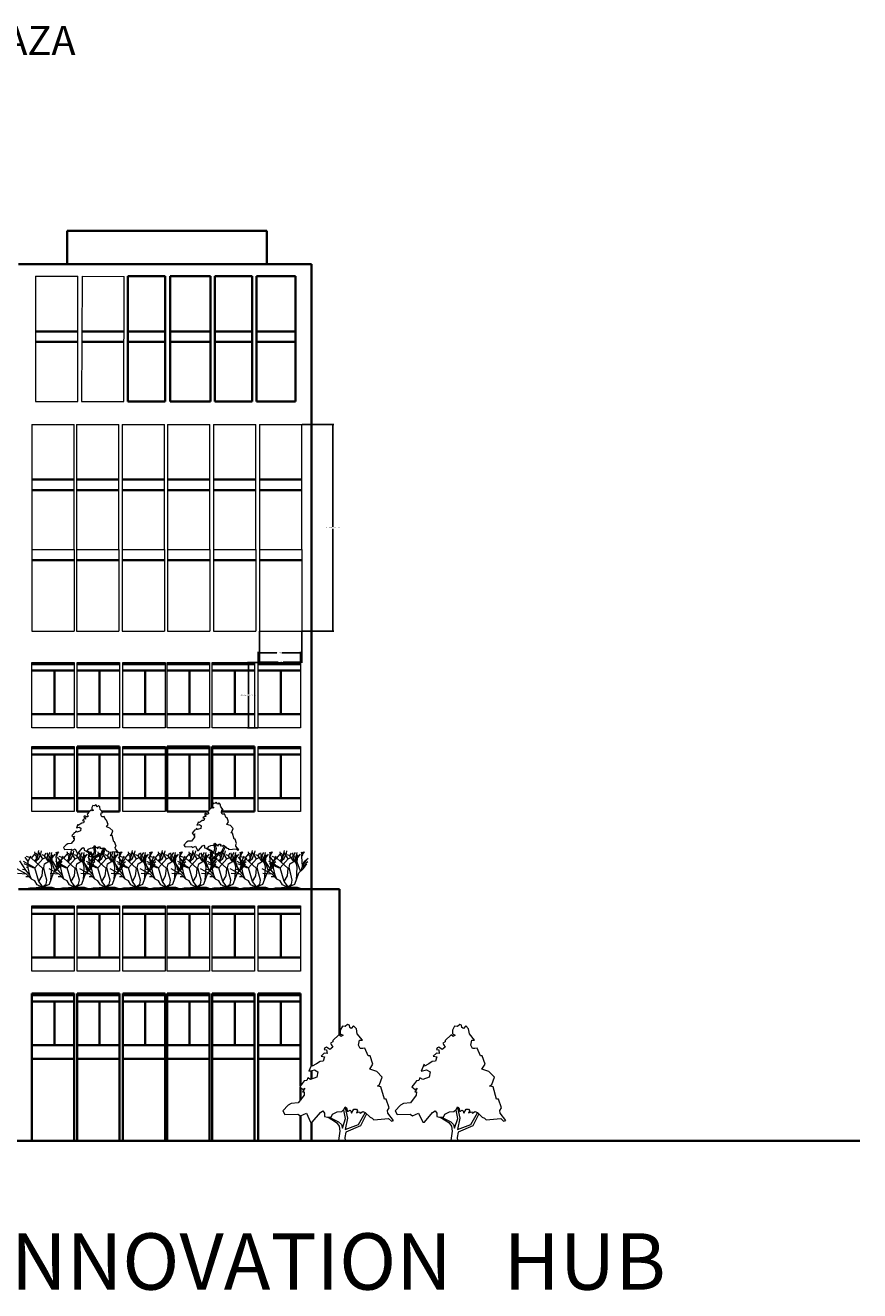
# Model space of a CAD drawing. Units: inches. Extents: x -362 to 223, y -437 to 70.
# Tile 5 of 5: x 67 to 223, y -166 to 70. Entities that reach past the tile are written whole.
import ezdxf

# ---------------------------------------------------------------- set-up
doc = ezdxf.new("R2010")
doc.units = ezdxf.units.IN
doc.header["$MEASUREMENT"] = 0
for name, color, linetype, lineweight in [('A-ANNO-DIMS', 2, 'Continuous', 18), ('A-ANNO-TEXT', 7, 'Continuous', 25), ('A-ELEV', 7, 'Continuous', 35), ('A-GLAZ', 4, 'Continuous', 18), ('L-PLNT', 3, 'Continuous', 13)]:
    doc.layers.add(name, color=color, linetype=linetype, lineweight=lineweight)
doc.styles.get("Standard").update_dxf_attribs({"font": 'arial.ttf'})
doc.dimstyles.get("Standard").update_dxf_attribs({"dimtxt": 0.18, "dimasz": 0.18, "dimexe": 0.18, "dimexo": 0.0625, "dimgap": 0.09, "dimtad": 0, "dimtih": 1, "dimtoh": 1, "dimdec": 4, "dimzin": 0, "dimdsep": 46, "dimtxsty": 'Standard', "dimcen": 0.09, "dimadec": 0, "dimazin": 0, "dimtfac": 1, "dimtdec": 4, "dimtofl": 0, "dimtmove": 0, "dimatfit": 3, "dimfxl": 1, "dimtolj": 1, "dimtzin": 0, "dimarcsym": 0})

# ---------------------------------------------------------------- blocks, each defined once
blk = doc.blocks.new('*U2')
for points in [[(22.0124, 137.721), (18.5475, 141.5624), (15.5282, 138.2446), (13.8028, 139.3505), (13.3714, 142.1153), (11.2148, 143.2214), (8.1954, 140.4564), (4.7447, 141.0094), (2.1567, 136.0326), (2.1567, 131.6088), (5.6074, 129.9499), (3.0193, 128.2909), (0.4313, 130.5029), (-6.9015, 123.3141), (-6.9015, 121.6552), (-9.9208, 119.9963), (-9.0581, 118.3373), (-6.9015, 115.0195), (-10.7835, 112.2546), (-14.6656, 115.0195), (-16.8222, 114.4665), (-17.6849, 112.2546), (-14.6656, 111.7016), (-14.2342, 107.2778), (-17.6065, 107.8307), (-21.5669, 103.9599), (-17.2536, 103.4069), (-18.9789, 97.8771), (-22.8609, 97.3241), (-27.1743, 94.5593), (-32.3504, 91.7944), (-32.7817, 94.0063), (-36.6638, 85.7116), (-29.7624, 87.3705), (-25.449, 84.6056), (-26.743, 77.9699), (-34.507, 75.205), (-37.9578, 77.4169), (-39.2518, 74.099), (-42.2711, 73.5461), (-44.8592, 70.2282), (-47.8786, 66.3574), (-43.9965, 63.0395), (-41.4085, 64.6985), (-44.3346, 59.8898), (-42.2089, 60.1377), (-42.5159, 55.7849), (-49.6039, 46.4502), (-58.2307, 45.8972), (-62.1127, 43.6853), (-68.5828, 36.4966), (-65.9947, 32.0727), (-50.0352, 32.6257), (-47.0159, 30.4138), (-39.6831, 33.7317), (-34.507, 22.6721), (-32.3504, 22.6721), (-22.4296, 34.8376), (-19.4102, 36.4966), (-17.2536, 33.7317), (-17.2536, 29.8608), (-13.8028, 28.7549), (-9.0581, 28.7549), (-7.3328, 32.6257), (-1.7254, 35.3906), (3.8821, 35.9436), (6.4701, 38.1555), (6.9014, 38.7085), (8.1954, 41.4734), (9.9208, 40.3674), (11.2148, 35.9436), (14.2341, 37.6025), (15.0968, 36.4966), (15.9595, 33.7317), (18.9789, 38.7085), (21.9982, 38.7085), (23.2922, 36.4966), (21.9982, 34.2847), (25.4489, 35.3906), (26.743, 33.7317), (29.7623, 35.9436), (32.7817, 34.8376), (38.8204, 28.7549), (41.4084, 27.6489), (43.5651, 25.437), (61.6813, 27.0959), (65.132, 23.7781), (67.7201, 24.884), (60.8186, 33.7317), (60.3873, 37.0495), (62.544, 40.3674), (58.662, 50.874), (56.5053, 50.874), (52.1919, 66.3574), (47.8785, 66.9103), (50.4665, 69.1222), (53.9172, 77.9699), (47.0158, 85.1586), (38.3891, 87.9235), (42.2711, 94.0063)], [(42.2711, 94.0063), (38.8204, 104.5129), (36.6637, 104.5129), (32.3503, 113.9135), (29.7623, 113.3605), (26.743, 113.3605), (24.5862, 117.7844), (25.8802, 123.8671), (29.331, 123.8671), (22.8609, 131.6088), (21.9982, 137.6916)], [(-9.9208, 28.2019), (0, 23.2251), (3.4507, 19.9072), (4.7447, 15.4834), (8.6267, 27.0959), (6.4701, 37.6025)], [(34.5071, 33.1787), (27.1743, 18.2483), (9.0581, 10.5066), (7.7641, 3.8708), (8.1954, 0)], [(8.1954, 40.3674), (11.2148, 27.6489), (8.1954, 13.8245), (24.5862, 19.9072), (32.7817, 34.2847)], [(-12.9401, 28.7549), (-2.588, 22.1191), (0.8626, 17.6953), (1.7253, 11.6125), (0, 0)]]:
    blk.add_lwpolyline(points)
blk = doc.blocks.new('*U4')
for p, q in [((-11.433, 18.289), (-10.457, 22.749)), ((-9.48, 19.775), (-8.992, 22.592)), ((-18.24, 11.04), (-21.755, 16.655)), ((-12.96, 12.48), (-19.68, 16.32)), ((-16.8, 16.32), (-18.72, 18.72)), ((-14.88, 18.24), (-17.76, 19.2)), ((-16.8, 16.32), (-15.36, 19.68)), ((-16.8, 12.48), (-16.8, 16.32)), ((-14.88, 18.24), (-12.96, 20.64)), ((-8.16, 12), (-14.88, 18.24)), ((-13.325, 16.724), (-11.433, 18.289)), ((-12.96, 12.48), (-8.16, 17.76)), ((-12.471, 19.775), (-12.898, 22.044)), ((-11.677, 19.071), (-12.471, 19.775)), ((-11.28, 19.619), (-12.104, 21.184)), ((-12.043, 15.628), (-11.921, 18.836)), ((-11.982, 16.802), (-10.579, 18.054)), ((-11.921, 18.836), (-10.64, 20.401)), ((-10.579, 18.054), (-9.846, 19.697)), ((-8.16, 17.76), (-10.56, 21.6)), ((-7.2, 19.68), (-8.64, 20.16)), ((-8.16, 17.76), (-5.28, 19.2)), ((-7.2, 19.68), (-6.24, 21.12)), ((-4.8, 16.32), (-7.2, 19.68)), ((-7.2, 14.88), (-3.84, 16.8)), ((-5.086, 17.741), (-5.513, 21.34)), ((-5.28, 19.2), (-3.84, 21.6)), ((-3.377, 15.315), (-5.086, 17.819)), ((-2.88, 12.96), (-4.32, 19.68)), ((-3.84, 16.8), (-0.96, 20.64)), ((-3.377, 18.602), (-2.888, 21.575)), ((-2.766, 16.802), (-3.377, 18.602)), ((-2.88, 15.84), (-2.4, 20.16)), ((-0.96, 10.56), (-2.88, 15.84)), ((-0.508, 21.888), (-0.081, 20.558)), ((-0.203, 19.149), (0.102, 21.34)), ((0.346, 13.203), (-0.203, 19.149)), ((-0.142, 19.384), (0.59, 20.401)), ((-0.02, 20.01), (0.896, 21.105)), ((0.041, 20.714), (1.384, 22.044)), ((0.102, 21.34), (0.835, 21.888)), ((0.346, 13.203), (1.323, 16.254)), ((0.96, 12), (1.44, 15.36)), ((1.323, 16.254), (3.642, 18.289)), ((1.44, 15.36), (2.88, 17.28)), ((1.92, 13.44), (2.4, 15.36)), ((2.4, 15.36), (3.36, 16.32)), ((-17.76, 8.64), (-23.663, 11.961)), ((-17.76, 8.64), (-23.128, 9.222)), ((-18.24, 11.04), (-20.16, 11.52)), ((-13.92, 12.48), (-19.2, 14.88)), ((-15.84, 8.16), (-18.24, 11.04)), ((-16.8, 12.48), (-17.76, 12.96)), ((-14.88, 5.76), (-17.76, 8.64)), ((-15.84, 8.16), (-16.8, 12.48)), ((-14.88, 5.76), (-15.84, 8.16)), ((-12.96, 12.48), (-13.92, 12.48)), ((-10.56, 4.32), (-12.96, 12.48)), ((-10.56, 4.32), (-8.64, 7.68)), ((-8.64, 7.68), (-8.16, 12)), ((-7.68, 12.48), (-7.2, 14.88)), ((-6.72, 8.64), (-7.68, 12.48)), ((-5.76, 5.28), (-6.72, 8.64)), ((-4.32, 2.88), (-1.92, 9.6)), ((-3.36, 5.28), (-2.88, 12.96)), ((-1.92, 9.6), (0.96, 12)), ((-0.48, 10.8), (0.346, 13.203)), ((0.96, 12), (2.88, 14.88)), ((-16.32, 7.2), (-18.24, 7.2)), ((-15.84, 0.48), (-17.76, 0)), ((-13.44, 0.48), (-15.84, 0.48)), ((-12.96, 4.8), (-14.88, 5.76)), ((-9.6, 0.96), (-13.44, 0.48)), ((-11.52, 2.4), (-12.96, 4.8)), ((-9.6, 0.96), (-12.96, 0)), ((-8.64, 0.96), (-11.52, 2.4)), ((-8.64, 1.92), (-10.56, 4.32)), ((-9.6, 0.96), (-7.68, 0.96)), ((-8.64, 0.96), (-4.32, 2.88)), ((-8.64, 0.96), (-6.24, 2.88)), ((-8.64, 0.96), (-8.64, 1.92)), ((-8.64, 0.96), (-2.88, 0.96)), ((-7.68, 0.96), (-6.24, 0.48)), ((-6.24, 2.88), (-5.76, 5.28)), ((-6.24, 0.48), (-3.36, 0)), ((-2.88, 0.96), (0, 0))]:
    blk.add_line(p, q)
blk = doc.blocks.new('WIN-PANEL-A')
for p, q in [((0, 12.16), (7.9, 12.16)), ((0, 0), (0, 12.16)), ((7.9, 12.16), (7.9, 0)), ((7.9, 0), (0, 0))]:
    blk.add_line(p, q)
blk = doc.blocks.new('WIN-TALL-A')
for p, q in [((0, 38.57), (7.9, 38.57)), ((0, 38.57), (0, 15.21)), ((0, 38.57), (7.9, 38.57)), ((7.9, 15.21), (7.9, 38.57)), ((0, 15.21), (7.9, 15.21)), ((0, 15.21), (0, 0)), ((7.9, 15.21), (7.9, 0)), ((0, 0), (7.9, 0))]:
    blk.add_line(p, q)
blk = doc.blocks.new('WIN-B')
for p, q in [((0, 23.36), (7.9, 23.36)), ((0, 23.36), (0, 0)), ((0, 23.36), (7.9, 23.36)), ((7.9, 0), (7.9, 23.36)), ((0, 0), (7.9, 0))]:
    blk.add_line(p, q)
blk = doc.blocks.new('*D15')
at = {"layer": 'A-ANNO-DIMS', "color": 0, "lineweight": -2, "transparency": 16777216}
for p, q in [((110.63, -48.56), (108.68, -48.56)), ((108.86, -48.74), (108.86, -54.46)), ((108.86, -60.54), (108.86, -54.83)), ((110.63, -60.72), (108.68, -60.72))]:
    blk.add_line(p, q, dxfattribs=at)
at = {"layer": 'A-ANNO-DIMS', "color": 0, "transparency": 16777216}
for points in [[(108.83, -48.74), (108.89, -48.74), (108.86, -48.56)], [(108.83, -60.54), (108.89, -60.54), (108.86, -60.72)]]:
    blk.add_solid(points, dxfattribs=at)
at = {"layer": 'Defpoints', "color": 0, "transparency": 16777216}
for p in [(110.69, -48.56), (108.86, -60.72), (110.69, -60.72)]:
    blk.add_point(p, dxfattribs=at)
at = {"layer": 'A-ANNO-DIMS', "color": 0, "transparency": 16777216, "insert": (108.86, -54.64), "char_height": 0.18, "attachment_point": 5}
blk.add_mtext('\\A1;WINDOW PANEL A 12 TYP.', dxfattribs=at)
blk = doc.blocks.new('*D16')
at = {"layer": 'A-ANNO-DIMS', "color": 0, "lineweight": -2, "transparency": 16777216}
for p, q in [((110.69, -48.5), (110.69, -46.56)), ((110.87, -46.74), (114.18, -46.74)), ((118.41, -46.74), (115.1, -46.74)), ((118.59, -48.5), (118.59, -46.56))]:
    blk.add_line(p, q, dxfattribs=at)
at = {"layer": 'A-ANNO-DIMS', "color": 0, "transparency": 16777216}
for points in [[(110.87, -46.71), (110.87, -46.77), (110.69, -46.74)], [(118.41, -46.71), (118.41, -46.77), (118.59, -46.74)]]:
    blk.add_solid(points, dxfattribs=at)
at = {"layer": 'Defpoints', "color": 0, "transparency": 16777216}
for p in [(110.69, -46.74), (110.69, -48.56), (118.59, -48.56)]:
    blk.add_point(p, dxfattribs=at)
at = {"layer": 'A-ANNO-DIMS', "color": 0, "transparency": 16777216, "insert": (114.64, -46.74), "char_height": 0.18, "attachment_point": 5}
blk.add_mtext('\\A1;8 TYP.', dxfattribs=at)
blk = doc.blocks.new('*D21')
at = {"layer": 'A-ANNO-DIMS', "color": 0, "lineweight": -2, "transparency": 16777216}
for p, q in [((118.91, -4.1), (124.81, -4.1)), ((124.63, -4.28), (124.63, -23.2)), ((124.63, -42.49), (124.63, -23.57)), ((118.91, -42.67), (124.81, -42.67))]:
    blk.add_line(p, q, dxfattribs=at)
at = {"layer": 'A-ANNO-DIMS', "color": 0, "transparency": 16777216}
for points in [[(124.6, -4.28), (124.66, -4.28), (124.63, -4.1)], [(124.6, -42.49), (124.66, -42.49), (124.63, -42.67)]]:
    blk.add_solid(points, dxfattribs=at)
at = {"layer": 'Defpoints', "color": 0, "transparency": 16777216}
for p in [(118.84, -4.1), (124.63, -4.1), (118.84, -42.67)]:
    blk.add_point(p, dxfattribs=at)
at = {"layer": 'A-ANNO-DIMS', "color": 0, "transparency": 16777216, "insert": (124.63, -23.38), "char_height": 0.18, "attachment_point": 5}
blk.add_mtext('\\A1;TALL WINDOW A 39 TYP.', dxfattribs=at)
blk = doc.blocks.new('*D22')
at = {"layer": 'A-ANNO-DIMS', "color": 0, "lineweight": -2, "transparency": 16777216}
for p, q in [((110.94, -42.73), (110.94, -48.64)), ((118.84, -42.73), (118.84, -48.64)), ((111.12, -48.46), (114.43, -48.46)), ((118.66, -48.46), (115.35, -48.46))]:
    blk.add_line(p, q, dxfattribs=at)
at = {"layer": 'A-ANNO-DIMS', "color": 0, "transparency": 16777216}
for points in [[(111.12, -48.43), (111.12, -48.49), (110.94, -48.46)], [(118.66, -48.43), (118.66, -48.49), (118.84, -48.46)]]:
    blk.add_solid(points, dxfattribs=at)
at = {"layer": 'Defpoints', "color": 0, "transparency": 16777216}
for p in [(110.94, -42.67), (118.84, -42.67), (118.84, -48.46)]:
    blk.add_point(p, dxfattribs=at)
at = {"layer": 'A-ANNO-DIMS', "color": 0, "transparency": 16777216, "insert": (114.89, -48.46), "char_height": 0.18, "attachment_point": 5}
blk.add_mtext('\\A1;8 TYP.', dxfattribs=at)

msp = doc.modelspace()

# ---------------------------------------------------------------- linework, layer by layer
at = {"layer": 'A-ELEV'}
for p, q in [((75.05, 25.83), (75.05, 32.03)), ((75.05, 32.03), (112.28, 32.03)), ((112.28, 32.03), (112.28, 25.83)), ((65.97, 25.83), (120.64, 25.83)), ((120.64, 25.83), (120.64, -1.59)), ((86.37, 0.18), (86.37, 23.54)), ((86.37, 23.54), (93.35, 23.54)), ((86.37, 23.54), (93.35, 23.54)), ((93.35, 0.18), (93.35, 23.54)), ((94.25, 0.18), (94.25, 23.54)), ((94.25, 23.54), (101.76, 23.54)), ((94.25, 23.54), (101.76, 23.54)), ((101.76, 0.18), (101.76, 23.54)), ((102.62, 0.18), (102.62, 23.54)), ((102.62, 23.54), (109.55, 23.54)), ((102.62, 23.54), (109.55, 23.54)), ((109.55, 0.18), (109.55, 23.54)), ((110.4, 0.18), (110.4, 23.54)), ((110.4, 23.54), (117.65, 23.54)), ((110.4, 23.54), (117.65, 23.54)), ((117.65, 23.54), (117.65, 0.18)), ((69.14, 13.22), (77.04, 13.22)), ((77.83, 13.22), (85.61, 13.22)), ((86.37, 13.22), (93.35, 13.22)), ((94.25, 13.22), (101.76, 13.22)), ((102.62, 13.22), (109.55, 13.22)), ((110.4, 13.22), (117.65, 13.22)), ((69.14, 11.29), (77.04, 11.29)), ((77.83, 11.29), (85.61, 11.29)), ((86.37, 11.29), (93.35, 11.29)), ((94.25, 11.29), (101.76, 11.29)), ((102.62, 11.29), (109.55, 11.29)), ((110.4, 11.29), (117.65, 11.29)), ((93.35, 0.18), (86.37, 0.18)), ((101.76, 0.18), (94.25, 0.18)), ((109.55, 0.18), (102.62, 0.18)), ((117.65, 0.18), (110.4, 0.18)), ((120.64, -1.59), (120.64, -57.83)), ((68.45, -14.42), (76.35, -14.42)), ((68.45, -16.35), (76.35, -16.35)), ((76.79, -14.42), (84.69, -14.42)), ((76.79, -16.35), (84.69, -16.35)), ((85.27, -14.42), (93.17, -14.42)), ((85.27, -16.35), (93.17, -16.35)), ((93.77, -14.42), (101.67, -14.42)), ((93.77, -16.35), (101.67, -16.35)), ((102.36, -14.42), (110.26, -14.42)), ((102.36, -16.35), (110.26, -16.35)), ((110.94, -14.42), (118.84, -14.42)), ((110.94, -16.35), (118.84, -16.35)), ((68.45, -29.46), (76.35, -29.46)), ((76.79, -29.46), (84.69, -29.46)), ((85.27, -29.46), (93.17, -29.46)), ((93.77, -29.46), (101.67, -29.46)), ((102.36, -29.46), (110.26, -29.46)), ((110.94, -29.46), (118.84, -29.46)), ((68.45, -48.88), (76.35, -48.88)), ((76.88, -48.88), (84.78, -48.88)), ((85.4, -48.88), (93.3, -48.88)), ((93.69, -48.88), (101.59, -48.88)), ((102.11, -48.88), (110.01, -48.88)), ((110.69, -48.88), (118.59, -48.88)), ((68.45, -50.04), (76.35, -50.04)), ((72.66, -58.19), (72.66, -50.04)), ((76.88, -50.04), (84.78, -50.04)), ((81.08, -58.19), (81.08, -50.04)), ((85.4, -50.04), (93.3, -50.04)), ((89.6, -58.19), (89.6, -50.04)), ((93.69, -50.04), (101.59, -50.04)), ((97.89, -58.19), (97.89, -50.04)), ((102.11, -50.04), (110.01, -50.04)), ((106.31, -58.19), (106.31, -50.04)), ((110.69, -50.04), (118.59, -50.04)), ((114.89, -58.19), (114.89, -50.04)), ((68.45, -58.19), (76.35, -58.19)), ((76.88, -58.19), (84.78, -58.19)), ((85.4, -58.19), (93.3, -58.19)), ((93.69, -58.19), (101.59, -58.19)), ((102.11, -58.19), (110.01, -58.19)), ((110.69, -58.19), (118.59, -58.19)), ((120.64, -57.83), (120.64, -103.71)), ((68.45, -64.55), (76.35, -64.55)), ((68.45, -65.7), (76.35, -65.7)), ((72.66, -73.85), (72.66, -65.7)), ((76.88, -64.23), (84.78, -64.23)), ((76.88, -76.39), (76.88, -64.23)), ((76.88, -64.55), (84.78, -64.55)), ((76.88, -65.7), (84.78, -65.7)), ((81.08, -73.85), (81.08, -65.7)), ((84.78, -64.23), (84.78, -76.39)), ((85.4, -64.55), (93.3, -64.55)), ((85.4, -65.7), (93.3, -65.7)), ((89.6, -73.85), (89.6, -65.7)), ((93.69, -64.23), (101.59, -64.23)), ((93.69, -76.39), (93.69, -64.23)), ((93.69, -64.55), (101.59, -64.55)), ((93.69, -65.7), (101.59, -65.7)), ((97.89, -73.85), (97.89, -65.7)), ((101.59, -64.23), (101.59, -75.98)), ((102.11, -64.23), (110.01, -64.23)), ((102.11, -75.67), (102.11, -64.23)), ((102.11, -64.55), (110.01, -64.55)), ((102.11, -65.7), (110.01, -65.7)), ((106.31, -73.85), (106.31, -65.7)), ((110.01, -64.23), (110.01, -76.39)), ((110.69, -64.55), (118.59, -64.55)), ((110.69, -65.7), (118.59, -65.7)), ((114.89, -73.85), (114.89, -65.7)), ((68.45, -73.85), (76.35, -73.85)), ((76.88, -73.85), (84.78, -73.85)), ((85.4, -73.85), (93.3, -73.85)), ((93.69, -73.85), (101.59, -73.85)), ((102.11, -73.85), (110.01, -73.85)), ((110.69, -73.85), (118.59, -73.85)), ((79.17, -76.39), (76.88, -76.39)), ((84.78, -76.39), (81.55, -76.39)), ((101.24, -76.39), (93.69, -76.39)), ((110.01, -76.39), (103.84, -76.39)), ((65.97, -90.83), (119.87, -90.83)), ((119.87, -90.83), (125.85, -90.83)), ((125.85, -90.83), (125.85, -118.1)), ((68.45, -94.3), (76.35, -94.3)), ((76.88, -94.3), (84.78, -94.3)), ((85.4, -94.3), (93.3, -94.3)), ((93.69, -94.3), (101.59, -94.3)), ((102.11, -94.3), (110.01, -94.3)), ((110.69, -94.3), (118.59, -94.3)), ((68.45, -95.46), (76.35, -95.46)), ((72.66, -103.6), (72.66, -95.46)), ((76.88, -95.46), (84.78, -95.46)), ((81.08, -103.6), (81.08, -95.46)), ((85.4, -95.46), (93.3, -95.46)), ((89.6, -103.6), (89.6, -95.46)), ((93.69, -95.46), (101.59, -95.46)), ((97.89, -103.6), (97.89, -95.46)), ((102.11, -95.46), (110.01, -95.46)), ((106.31, -103.6), (106.31, -95.46)), ((110.69, -95.46), (118.59, -95.46)), ((114.89, -103.6), (114.89, -95.46)), ((68.45, -103.6), (76.35, -103.6)), ((76.88, -103.6), (84.78, -103.6)), ((85.4, -103.6), (93.3, -103.6)), ((93.69, -103.6), (101.59, -103.6)), ((102.11, -103.6), (110.01, -103.6)), ((110.69, -103.6), (118.59, -103.6)), ((120.64, -123.72), (120.64, -103.71)), ((68.45, -110.34), (76.35, -110.34)), ((68.45, -137.85), (68.45, -110.34)), ((68.45, -110.66), (76.35, -110.66)), ((76.35, -110.34), (76.35, -137.85)), ((76.88, -110.34), (84.78, -110.34)), ((76.88, -137.85), (76.88, -110.34)), ((76.88, -110.66), (84.78, -110.66)), ((84.78, -110.34), (84.78, -137.85)), ((85.4, -110.34), (93.3, -110.34)), ((85.4, -137.85), (85.4, -110.34)), ((85.4, -110.66), (93.3, -110.66)), ((93.3, -110.34), (93.3, -137.85)), ((93.69, -110.34), (101.59, -110.34)), ((93.69, -137.85), (93.69, -110.34)), ((93.69, -110.66), (101.59, -110.66)), ((101.59, -110.34), (101.59, -137.85)), ((102.11, -110.34), (110.01, -110.34)), ((102.11, -137.85), (102.11, -110.34)), ((102.11, -110.66), (110.01, -110.66)), ((110.01, -110.34), (110.01, -137.85)), ((110.69, -110.34), (118.59, -110.34)), ((110.69, -137.85), (110.69, -110.34)), ((110.69, -110.66), (118.59, -110.66)), ((118.59, -110.34), (118.59, -127.54)), ((68.45, -111.81), (76.35, -111.81)), ((72.66, -119.96), (72.66, -111.81)), ((76.88, -111.81), (84.78, -111.81)), ((81.08, -119.96), (81.08, -111.81)), ((85.4, -111.81), (93.3, -111.81)), ((89.6, -119.96), (89.6, -111.81)), ((93.69, -111.81), (101.59, -111.81)), ((97.89, -119.96), (97.89, -111.81)), ((102.11, -111.81), (110.01, -111.81)), ((106.31, -119.96), (106.31, -111.81)), ((110.69, -111.81), (118.59, -111.81)), ((114.89, -119.96), (114.89, -111.81)), ((68.45, -119.96), (76.35, -119.96)), ((76.88, -119.96), (84.78, -119.96)), ((85.4, -119.96), (93.3, -119.96)), ((93.69, -119.96), (101.59, -119.96)), ((102.11, -119.96), (110.01, -119.96)), ((110.69, -119.96), (118.59, -119.96)), ((76.35, -122.5), (68.45, -122.5)), ((84.78, -122.5), (76.88, -122.5)), ((93.3, -122.5), (85.4, -122.5)), ((101.59, -122.5), (93.69, -122.5)), ((110.01, -122.5), (102.11, -122.5)), ((118.59, -122.5), (110.69, -122.5)), ((120.64, -126.33), (120.64, -124.68)), ((118.59, -127.87), (118.59, -130.21)), ((118.59, -133.17), (118.59, -137.85)), ((120.64, -137.85), (120.64, -134.36)), ((-11.78, -137.85), (200.92, -137.85)), ((65.97, -137.85), (119.87, -137.85)), ((125.85, -137.85), (119.87, -137.85)), ((200.92, -137.85), (222.98, -137.85))]:
    msp.add_line(p, q, dxfattribs=at)

# ---------------------------------------------------------------- block references
at = {"layer": 'A-GLAZ'}
for name, p in [('WIN-B', (69.14, 0.18)), ('WIN-TALL-A', (68.45, -42.67)), ('WIN-TALL-A', (76.79, -42.67)), ('WIN-TALL-A', (85.27, -42.67)), ('WIN-TALL-A', (93.77, -42.67)), ('WIN-TALL-A', (102.36, -42.67)), ('WIN-TALL-A', (110.94, -42.67)), ('WIN-PANEL-A', (68.45, -60.72))]:
    msp.add_blockref(name, p, dxfattribs=at)
for name, p, rotation in [('WIN-B', (77.69, 0.2), 359.7442576066927), ('WIN-PANEL-A', (84.78, -48.56), 180), ('WIN-PANEL-A', (93.3, -48.56), 180), ('WIN-PANEL-A', (101.59, -48.56), 180), ('WIN-PANEL-A', (110.01, -48.56), 180), ('WIN-PANEL-A', (118.59, -48.56), 180), ('WIN-PANEL-A', (76.35, -64.23), 180), ('WIN-PANEL-A', (93.3, -64.23), 180), ('WIN-PANEL-A', (118.59, -64.23), 180), ('WIN-PANEL-A', (76.35, -93.98), 180), ('WIN-PANEL-A', (84.78, -93.98), 180), ('WIN-PANEL-A', (93.3, -93.98), 180), ('WIN-PANEL-A', (101.59, -93.98), 180), ('WIN-PANEL-A', (110.01, -93.98), 180), ('WIN-PANEL-A', (118.59, -93.98), 180)]:
    msp.add_blockref(name, p, dxfattribs=dict(at, rotation=rotation))
at = {"layer": 'L-PLNT'}
for name, p, xscale, yscale, zscale in [('*U2', (79.49, -85.83), 0.0749300407806004, 0.0749300407806004, 0.0749300407806004), ('*U2', (101.97, -85.36), 0.0749300407806004, 0.0749300407806004, 0.0749300407806004), ('*U4', (73.06, -90.81), 0.3151431067188808, 0.3151431067188808, 0.3151431067188808), ('*U4', (79.12, -90.81), 0.3151431067188808, 0.3151431067188808, 0.3151431067188808), ('*U4', (84.85, -90.81), 0.3151431067188808, 0.3151431067188808, 0.3151431067188808), ('*U4', (90.53, -90.81), 0.3151431067188808, 0.3151431067188808, 0.3151431067188808), ('*U4', (96.13, -90.81), 0.3151431067188808, 0.3151431067188808, 0.3151431067188808), ('*U4', (101.87, -90.81), 0.3151431067188808, 0.3151431067188808, 0.3151431067188808), ('*U4', (107.4, -90.81), 0.3151431067188808, 0.3151431067188808, 0.3151431067188808), ('*U4', (112.94, -90.81), 0.3151431067188808, 0.3151431067188808, 0.3151431067188808), ('*U4', (118.87, -90.81), 0.3151431067188808, 0.3151431067188808, 0.3151431067188808), ('*U2', (125.69, -137.79), 0.1515196865409096, 0.1515196865409096, 0.1515196865409096), ('*U2', (146.64, -137.79), 0.1515196865409096, 0.1515196865409096, 0.1515196865409096)]:
    msp.add_blockref(name, p, dxfattribs=dict(at, xscale=xscale, yscale=yscale, zscale=zscale))

# ---------------------------------------------------------------- texts
at = {"layer": 'A-ANNO-TEXT'}
for s, height, p in [('STUDENT   PLAZA', 5.4377, (15.9, 64.85)), ('PRIMARY   CAMPUS  AXIS   ELEVATION   STUDENT  UNION   AND   INNOVATION   HUB ', 10.5337, (-363.29, -165.62))]:
    msp.add_text(s, height=height, dxfattribs=at).set_placement(p)

# ---------------------------------------------------------------- dimensions: what is measured, and where the dimension line sits
at = {"layer": 'A-ANNO-DIMS'}
for base, p1, p2, angle, text, picture, middle in [((124.63, -4.1), (118.84, -42.67), (118.84, -4.1), 90, 'TALL WINDOW A <> TYP.', '*D21', (124.63, -23.38)), ((110.69, -46.74), (118.59, -48.56), (110.69, -48.56), 180, '<> TYP.', '*D16', (114.64, -46.74)), ((108.86, -60.72), (110.69, -48.56), (110.69, -60.72), 270, 'WINDOW PANEL A <> TYP.', '*D15', (108.86, -54.64))]:
    dim = msp.add_linear_dim(base=base, p1=p1, p2=p2, angle=angle, text=text, dimstyle='Standard', override={"dimdec": 0, "dimlfac": 1, "dimrnd": 0, "dimzin": 0, "dimdsep": 46, "dimlunit": 2}, dxfattribs=at)
    dim.commit()
    dim.dimension.update_dxf_attribs({"geometry": picture, "text_midpoint": middle})
dim = msp.add_linear_dim(base=(118.84, -48.46), p1=(110.94, -42.67), p2=(118.84, -42.67), text='<> TYP.', dimstyle='Standard', override={"dimdec": 0, "dimlfac": 1, "dimrnd": 0, "dimzin": 0, "dimdsep": 46, "dimlunit": 2}, dxfattribs=at)
dim.commit()
dim.dimension.update_dxf_attribs({"geometry": '*D22', "text_midpoint": (114.89, -48.46)})

doc.saveas('drawing.dxf')
